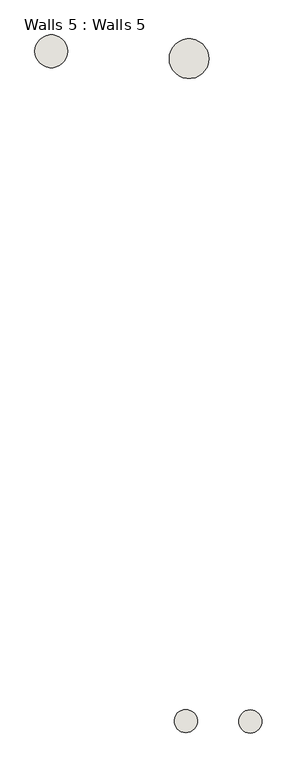
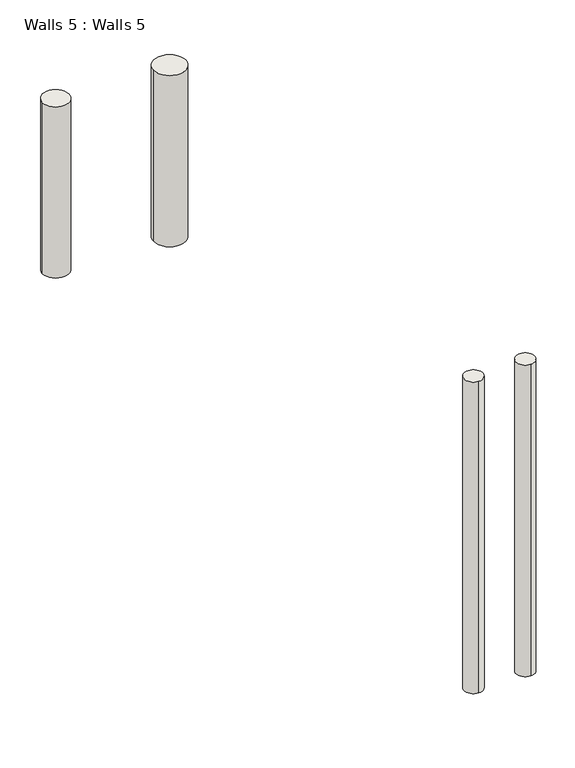
"""IFC4 building model written with IfcOpenShell, lengths in millimetres: wall geometry, Walls 5 : Walls 5."""

from ifc_helpers import new_model, si_unit, point, frame, frame_2d, origin, place, context, project, spatial, circle_curve, trimmed, segment, composite_curve, outline, extrude, source, transform, mapped, element, save


def walls_5_walls_5_b947fde3(model_context):
    return source(origin(), model_context, "Body", "SweptSolid", [
        extrude(outline(composite_curve([segment(trimmed(circle_curve(frame_2d((121.9670786, 7474.0998712)), 252.2580065), [point((-130.2909279, 7474.0998712))], [point((374.2250851, 7474.0998712))], False, "CARTESIAN"), True, "CONTINUOUS"), segment(trimmed(circle_curve(frame_2d((121.9670786, 7474.0998712)), 252.2580065), [point((374.2250851, 7474.0998712))], [point((-130.2909279, 7474.0998712))], False, "CARTESIAN"), True, "CONTINUOUS")], self_intersect=False)), frame((0.0, 0.0, 14935.2), z_axis=(0.0, 0.0, 1.0), x_axis=(1.0, 0.0, 0.0)), (0.0, 0.0, 1.0), 3466.8507068),
        extrude(outline(composite_curve([segment(trimmed(circle_curve(frame_2d((2241.6506935, 7359.7940802)), 304.8), [point((1936.8506935, 7359.7940802))], [point((2546.4506935, 7359.7940802))], False, "CARTESIAN"), True, "CONTINUOUS"), segment(trimmed(circle_curve(frame_2d((2241.6506935, 7359.7940802)), 304.8), [point((2546.4506935, 7359.7940802))], [point((1936.8506935, 7359.7940802))], False, "CARTESIAN"), True, "CONTINUOUS")], self_intersect=False)), frame((0.0, 0.0, 14935.2), z_axis=(0.0, 0.0, 1.0), x_axis=(1.0, 0.0, 0.0)), (0.0, 0.0, 1.0), 3466.8507068),
        extrude(outline(composite_curve([segment(trimmed(circle_curve(frame_2d((2190.6090714, -2809.8999415)), 177.8), [point((2190.6090714, -2987.6999415))], [point((2190.6090714, -2632.0999415))], False, "CARTESIAN"), True, "CONTINUOUS"), segment(trimmed(circle_curve(frame_2d((2190.6090714, -2809.8999415)), 177.8), [point((2190.6090714, -2632.0999415))], [point((2190.6090714, -2987.6999415))], False, "CARTESIAN"), True, "CONTINUOUS")], self_intersect=False)), frame((0.0, 0.0, 11976.102518), z_axis=(0.0, 0.0, 1.0), x_axis=(1.0, 0.0, 0.0)), (0.0, 0.0, 1.0), 6311.897482),
        extrude(outline(composite_curve([segment(trimmed(circle_curve(frame_2d((3181.3455808, -2815.1632065)), 177.8), [point((3181.3455808, -2992.9632065))], [point((3181.3455808, -2637.3632065))], False, "CARTESIAN"), True, "CONTINUOUS"), segment(trimmed(circle_curve(frame_2d((3181.3455808, -2815.1632065)), 177.8), [point((3181.3455808, -2637.3632065))], [point((3181.3455808, -2992.9632065))], False, "CARTESIAN"), True, "CONTINUOUS")], self_intersect=False)), frame((0.0, 0.0, 11976.102518), z_axis=(0.0, 0.0, 1.0), x_axis=(1.0, 0.0, 0.0)), (0.0, 0.0, 1.0), 6311.897482),
    ])


if __name__ == "__main__":
    model = new_model("IFC4")
    model_context = context("Model", 3, world=origin())
    ifc_project = project(units=[si_unit("LENGTHUNIT", "METRE", prefix="MILLI")], contexts=[model_context])
    site = spatial("IfcSite", under=ifc_project)
    building = spatial("IfcBuilding", under=site)
    placement = place(None, origin())
    walls_5_walls_5_shape = walls_5_walls_5_b947fde3(model_context)
    element("IfcWall", 1, ObjectType="Walls 5 : Walls 5", at=placement, inside=building, context=model_context, shape_type="MappedRepresentation", body=[
        mapped(walls_5_walls_5_shape, transform((0.0, 0.0, 0.0), x_axis=(1.0, 0.0, 0.0), y_axis=(0.0, 1.0, 0.0), z_axis=(0.0, 0.0, 1.0))),
    ])
    save(model, "model.ifc")

# Revit data of these elements
# Element 1 (IfcWall, "Walls 5 : Walls 5")
#   Materials on its faces: "Default Wall"
# Materials
#   "Default Wall": colour RGB 128 128 128, transparency 0
